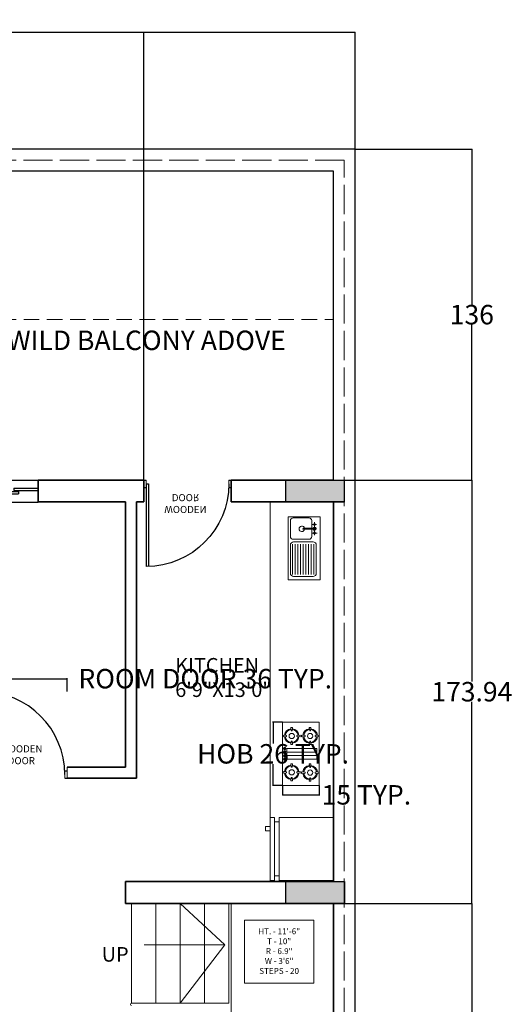
# Model space of a CAD drawing. Units: inches. Extents: x -48 to 50072, y 0 to 21068.
# Tile 56 of 75: x 415 to 618, y 819 to 1224. Entities that reach past the tile are written whole.
import ezdxf

# ---------------------------------------------------------------- set-up
doc = ezdxf.new("R2010")
doc.units = ezdxf.units.IN
doc.header["$MEASUREMENT"] = 0
doc.linetypes.add('ACAD_ISO02W100', pattern=[15, 12, -3])
doc.linetypes.add('HIDDEN', pattern=[9.525, 6.35, -3.175])
for name, color, linetype, lineweight in [('A-ANNO-DIMS', 2, 'Continuous', 18), ('A-ANNO-SYMB', 7, 'Continuous', 18), ('A-ANNO-TEXT', 7, 'Continuous', 18), ('A-AREA-IDEN', 7, 'Continuous', 18), ('A-COLS', 1, 'Continuous', 35), ('A-DOOR', 4, 'Continuous', 18), ('A-EQPM', 8, 'Continuous', 18), ('A-FLOR-CASE', 9, 'Continuous', 18), ('A-FLOR-FIXT', 4, 'Continuous', 18), ('A-FLOR-OVHD', 8, 'HIDDEN', 13), ('A-FLOR-STRS', 7, 'Continuous', 18), ('A-GLAZ', 4, 'Continuous', 18), ('A-WALL', 7, 'Continuous', 35), ('C-PROP', 7, 'Continuous', 25), ('C-PROP-REF', 32, 'ACAD_ISO02W100', 13)]:
    doc.layers.add(name, color=color, linetype=linetype, lineweight=lineweight)
doc.layers.add('Layer3', color=176, linetype='Continuous')
doc.styles.get("Standard").update_dxf_attribs({"font": 'arial.ttf'})
doc.dimstyles.get("Standard").update_dxf_attribs({"dimtxt": 8, "dimasz": 0.18, "dimexe": 0.18, "dimexo": 0.0625, "dimgap": 0.09, "dimtad": 0, "dimtih": 1, "dimtoh": 1, "dimdec": 1, "dimzin": 0, "dimdsep": 46, "dimlunit": 4, "dimtxsty": 'Standard', "dimblk": 'ARCHTICK', "dimcen": 0.09, "dimadec": 0, "dimazin": 0, "dimtfac": 1, "dimtdec": 1, "dimtofl": 0, "dimtmove": 0, "dimatfit": 3, "dimldrblk": 'ARCHTICK', "dimfxl": 1, "dimtolj": 1, "dimtzin": 0, "dimarcsym": 0})

# ---------------------------------------------------------------- blocks, each defined once
blk = doc.blocks.new('bnniku')
at = {"layer": 'Defpoints'}
h = blk.add_hatch(color=256, dxfattribs=at)
h.dxf.hatch_style = 1
h.paths.add_polyline_path([(767.55, 1114.04), (758.55, 1114.04), (758.55, 1090.04), (767.55, 1090.04)])
for p, q in [((758.55, 1114.04), (767.55, 1114.04)), ((758.55, 1090.04), (758.55, 1114.04)), ((767.55, 1114.04), (767.55, 1090.04)), ((767.55, 1090.04), (758.55, 1090.04))]:
    blk.add_line(p, q, dxfattribs=at)
blk = doc.blocks.new('jyugcli')
for p, q in [((342.02, 1025.77), (342.02, 1034.77)), ((360.02, 1025.77), (360.02, 1034.77))]:
    blk.add_line(p, q)
at = {"layer": 'Defpoints'}
for p, q in [((342.02, 1030.07), (352.02, 1030.07)), ((342.02, 1029.07), (352.02, 1029.07)), ((350.02, 1031.47), (360.02, 1031.47)), ((350.02, 1031.47), (350.02, 1030.47)), ((350.02, 1030.47), (360.02, 1030.47)), ((352.02, 1030.07), (352.02, 1029.07))]:
    blk.add_line(p, q, dxfattribs=at)
at = {"layer": 'Layer3'}
for p, q in [((342.02, 1034.77), (360.02, 1034.77)), ((342.02, 1025.77), (360.02, 1025.77))]:
    blk.add_line(p, q, dxfattribs=at)
blk = doc.blocks.new('BKUHJKKUG')
at = {"layer": 'Defpoints'}
for p, q in [((179.52, 862.77), (179.52, 896.77)), ((180.52, 862.77), (180.52, 896.76)), ((179.52, 862.77), (180.52, 862.77))]:
    blk.add_line(p, q, dxfattribs=at)
blk.add_arc((179.52, 862.77), 34, 0, 90, dxfattribs=at)
at = {"insert": (190.84, 874.8), "char_height": 2.9183, "attachment_point": 1}
blk.add_mtext_dynamic_manual_height_columns('\\pxqc;WOODEN ^JDOOR', width=9.6242, gutter_width=14.59, heights=[0], dxfattribs=at)
blk = doc.blocks.new('yfhjudru')
for p, q in [((399.02, 912.27), (399.02, 916.77)), ((400.02, 912.27), (400.02, 915.27)), ((434.02, 912.27), (434.02, 915.27)), ((435.02, 912.27), (435.02, 916.77))]:
    blk.add_line(p, q)
at = {"layer": 'Defpoints'}
for p, q in [((399.02, 915.27), (400.02, 915.27)), ((434.02, 915.27), (435.02, 915.27)), ((399.02, 912.27), (400.02, 912.27)), ((434.02, 912.27), (435.02, 912.27))]:
    blk.add_line(p, q, dxfattribs=at)
blk.add_blockref('BKUHJKKUG', (220.5, 51), dxfattribs=at)
blk = doc.blocks.new('A$C593E77E4')
for p, q in [((0, 0), (0, 0.911)), ((0, 0.911), (1.781, 0.911)), ((1.781, 0), (1.781, 0.911)), ((0.03, 0.593), (0.03, 0.141)), ((0.321, 0.668), (0.105, 0.668)), ((0.279, 0.745, -0.922), (0.15, 0.745, -0.922)), ((0.216, 0.808, -0.922), (0.216, 0.672, -0.922)), ((0.321, 0.784, -0.922), (0.321, 0.434, -0.922)), ((0.349, 0.784, -0.922), (0.321, 0.784, -0.922)), ((0.349, 0.434, -0.922), (0.349, 0.784, -0.922)), ((0.555, 0.668), (0.349, 0.668)), ((0.39, 0.745, -0.922), (0.519, 0.745, -0.922)), ((0.455, 0.826, -0.922), (0.455, 0.689, -0.922)), ((0.63, 0.141), (0.63, 0.593)), ((0.705, 0.706), (0.705, 0.158)), ((0.772, 0.729, 1.373), (1.625, 0.729, 1.373)), ((0.772, 0.654, 1.373), (1.625, 0.654, 1.373)), ((0.772, 0.579, 1.373), (1.625, 0.579, 1.373)), ((1.588, 0.797), (0.797, 0.797)), ((1.68, 0.158), (1.68, 0.706)), ((0.772, 0.504, 1.373), (1.625, 0.504, 1.373)), ((0.772, 0.429, 1.373), (1.625, 0.429, 1.373)), ((0.772, 0.354, 1.373), (1.625, 0.354, 1.373)), ((0.772, 0.279, 1.373), (1.625, 0.279, 1.373)), ((0.105, 0.066), (0.555, 0.066)), ((0.772, 0.204, 1.373), (1.625, 0.204, 1.373)), ((0.772, 0.129, 1.373), (1.625, 0.129, 1.373)), ((0.797, 0.066), (1.588, 0.066)), ((1.781, 0), (0, 0))]:
    blk.add_line(p, q)
for centre in [(0.216, 0.745, -0.922), (0.454, 0.745, -0.922)]:
    blk.add_circle(centre, 0.0299)
for centre, radius, start, end in [((0.105, 0.593), 0.075, 90, 180), ((0.333, 0.75, -0.922), 0.0447, 290.1713, 253.9866), ((0.555, 0.593), 0.075, 0, 90), ((0.797, 0.706), 0.0919, 90, 180), ((1.588, 0.706), 0.0919, 0, 90), ((0.336, 0.387, 0.688), 0.0774, 101.239, 83.3158), ((0.335, 0.435, -0.922), 0.0139, 185.1203, 354.8797), ((0.105, 0.141), 0.075, 180, 270), ((0.555, 0.141), 0.075, 270, 0), ((0.797, 0.158), 0.0919, 180, 270), ((1.588, 0.158), 0.0919, 270, 0)]:
    blk.add_arc(centre, radius, start, end)
blk = doc.blocks.new('A$C57CF26DA')
for p, q in [((0, 0), (0, 420)), ((720, 420), (0, 420)), ((167, 413), (147, 413)), ((147, 413), (152, 373)), ((152, 373), (162, 373)), ((162, 373), (167, 413)), ((300, 391), (300, 49)), ((300, 391), (420, 391)), ((340, 391), (340, 49)), ((380, 391), (380, 49)), ((420, 391), (420, 49)), ((584, 413), (564, 413)), ((564, 413), (569, 373)), ((569, 373), (579, 373)), ((579, 373), (584, 413)), ((720, 0), (720, 420)), ((99, 320), (59, 325)), ((59, 325), (59, 305)), ((59, 305), (99, 310)), ((99, 310), (99, 320)), ((152, 257), (147, 217)), ((162, 257), (152, 257)), ((167, 217), (162, 257)), ((255, 325), (215, 320)), ((215, 320), (215, 310)), ((215, 310), (255, 305)), ((255, 305), (255, 325)), ((516, 320), (476, 325)), ((476, 325), (476, 305)), ((476, 305), (516, 310)), ((516, 310), (516, 320)), ((569, 257), (564, 217)), ((579, 257), (569, 257)), ((584, 217), (579, 257)), ((672, 325), (632, 320)), ((632, 320), (632, 310)), ((632, 310), (672, 305)), ((672, 305), (672, 325)), ((99, 110), (59, 115)), ((59, 115), (59, 95)), ((147, 217), (167, 217)), ((167, 203), (147, 203)), ((147, 203), (152, 163)), ((152, 163), (162, 163)), ((162, 163), (167, 203)), ((255, 115), (215, 110)), ((255, 95), (255, 115)), ((513, 110), (473, 115)), ((473, 115), (473, 95)), ((581, 203), (561, 203)), ((561, 203), (566, 163)), ((564, 217), (584, 217)), ((566, 163), (576, 163)), ((576, 163), (581, 203)), ((669, 115), (629, 110)), ((669, 95), (669, 115)), ((59, 95), (99, 100)), ((99, 100), (99, 110)), ((152, 47), (147, 7)), ((147, 7), (167, 7)), ((162, 47), (152, 47)), ((167, 7), (162, 47)), ((215, 110), (215, 100)), ((215, 100), (255, 95)), ((302, 39), (295, 39)), ((295, 39), (295, 11)), ((295, 11), (302, 11)), ((420, 49), (300, 49)), ((302, 11), (302, 39)), ((341, 39), (334, 39)), ((334, 39), (334, 11)), ((334, 11), (341, 11)), ((341, 11), (341, 39)), ((380, 11), (380, 39)), ((380, 39), (386, 39)), ((386, 11), (380, 11)), ((386, 39), (386, 11)), ((419, 11), (419, 39)), ((419, 39), (426, 39)), ((426, 11), (419, 11)), ((426, 39), (426, 11)), ((473, 95), (513, 100)), ((513, 100), (513, 110)), ((566, 47), (561, 7)), ((561, 7), (581, 7)), ((576, 47), (566, 47)), ((581, 7), (576, 47)), ((629, 110), (629, 100)), ((629, 100), (669, 95)), ((720, 0), (0, 0))]:
    blk.add_line(p, q)
for centre in [(157, 315), (574, 315), (157, 105), (571, 105)]:
    blk.add_circle(centre, 30)
for centre, radius, start, end in [((157, 315), 83, 95.5849, 174.4151), ((157, 315), 73, 95.3738, 174.6262), ((157, 315), 73, 5.3738, 84.6262), ((157, 315), 83, 5.5849, 84.4151), ((574, 315), 83, 95.5849, 174.4151), ((574, 315), 73, 95.3738, 174.6262), ((574, 315), 73, 5.3738, 84.6262), ((574, 315), 83, 5.5849, 84.4151), ((157, 315), 83, 185.5849, 264.4151), ((157, 315), 73, 185.3738, 264.6262), ((157, 315), 73, 275.3738, 354.6262), ((157, 315), 83, 275.5849, 354.4151), ((574, 315), 83, 185.5849, 264.4151), ((574, 315), 73, 185.3738, 264.6262), ((574, 315), 73, 275.3738, 354.6262), ((574, 315), 83, 275.5849, 354.4151), ((157, 105), 83, 95.5849, 174.4151), ((157, 105), 73, 95.3738, 174.6262), ((157, 105), 73, 5.3738, 84.6262), ((157, 105), 83, 5.5849, 84.4151), ((571, 105), 83, 95.5849, 174.4151), ((571, 105), 73, 95.3738, 174.6262), ((571, 105), 73, 5.3738, 84.6262), ((571, 105), 83, 5.5849, 84.4151), ((157, 105), 83, 185.5849, 264.4151), ((157, 105), 73, 185.3738, 264.6262), ((157, 105), 73, 275.3738, 354.6262), ((157, 105), 83, 275.5849, 354.4151), ((298, 25), 13.7, 104.4775, 255.5225), ((298, 25), 13.7, 284.4775, 75.5225), ((337, 25), 13.7, 104.4775, 255.5225), ((337, 25), 13.7, 284.4775, 75.5225), ((383, 25), 13.7, 104.4775, 255.5225), ((383, 25), 13.7, 284.4775, 75.5225), ((422, 25), 13.7, 104.4775, 255.5225), ((422, 25), 13.7, 284.4775, 75.5225), ((571, 105), 83, 185.5849, 264.4151), ((571, 105), 73, 185.3738, 264.6262), ((571, 105), 73, 275.3738, 354.6262), ((571, 105), 83, 275.5849, 354.4151)]:
    blk.add_arc(centre, radius, start, end)
blk = doc.blocks.new('REFRI-00')
for points in [[(-0.35, 0.35), (-0.35, -0.25), (0.35, -0.25), (0.35, 0.35), (-0.35, 0.35)], [(-0.35, -0.3), (-0.35, -0.35), (0.35, -0.35), (0.35, -0.3), (-0.35, -0.3)], [(-0.3, -0.3), (-0.3, -0.25)], [(0.3, -0.3), (0.3, -0.25)], [(-0.25, -0.35), (-0.25, -0.4), (-0.2, -0.4), (-0.2, -0.35)]]:
    blk.add_lwpolyline(points)
blk = doc.blocks.new('_ArchTick')
at = {"color": 0, "linetype": 'ByBlock', "const_width": 0.15}
blk.add_lwpolyline([(-0.5, -0.5), (0.5, 0.5)], dxfattribs=at)
blk = doc.blocks.new('*D64')
at = {"layer": 'A-ANNO-DIMS', "color": 0, "lineweight": -2, "transparency": 16777216}
for p, q in [((399.02, 947.84), (399.02, 953.35)), ((399.02, 953.17), (435.02, 953.17)), ((435.02, 947.84), (435.02, 953.35)), ((435.02, 953.17), (435.2, 953.17))]:
    blk.add_line(p, q, dxfattribs=at)
at = {"layer": 'Defpoints', "color": 0, "transparency": 16777216}
for p in [(435.02, 953.17), (399.02, 947.77), (435.02, 947.77)]:
    blk.add_point(p, dxfattribs=at)
at = {"layer": 'A-ANNO-DIMS', "color": 0, "lineweight": -2, "transparency": 16777216, "xscale": 0.18, "yscale": 0.18, "zscale": 0.18, "rotation": 180}
blk.add_blockref('_ArchTick', (399.02, 953.17), dxfattribs=at)
at = {"layer": 'A-ANNO-DIMS', "color": 0, "lineweight": -2, "transparency": 16777216, "xscale": 0.18, "yscale": 0.18, "zscale": 0.18}
blk.add_blockref('_ArchTick', (435.02, 953.17), dxfattribs=at)
at = {"layer": 'A-ANNO-DIMS', "color": 0, "transparency": 16777216, "insert": (491.8, 953.17), "char_height": 8, "attachment_point": 5}
blk.add_mtext('\\A1;ROOM DOOR 36 TYP.', dxfattribs=at)
blk = doc.blocks.new('*D90')
at = {"layer": 'A-ANNO-DIMS', "color": 0, "lineweight": -2, "transparency": 16777216}
for p, q in [((523.53, 935.26), (519.52, 935.26)), ((519.7, 935.26), (519.7, 926.52)), ((519.7, 909.32), (519.7, 918.06)), ((523.53, 909.32), (519.52, 909.32))]:
    blk.add_line(p, q, dxfattribs=at)
at = {"layer": 'Defpoints', "color": 0, "transparency": 16777216}
for p in [(523.59, 935.26), (519.7, 909.32), (523.59, 909.32)]:
    blk.add_point(p, dxfattribs=at)
at = {"layer": 'A-ANNO-DIMS', "color": 0, "lineweight": -2, "transparency": 16777216, "xscale": 0.18, "yscale": 0.18, "zscale": 0.18}
for p, rotation in [((519.7, 935.26), 90), ((519.7, 909.32), 270)]:
    blk.add_blockref('_ArchTick', p, dxfattribs=dict(at, rotation=rotation))
at = {"layer": 'A-ANNO-DIMS', "color": 0, "transparency": 16777216, "insert": (519.7, 922.29), "char_height": 8, "attachment_point": 5}
blk.add_mtext('\\A1;HOB 26 TYP.', dxfattribs=at)
blk = doc.blocks.new('*D91')
at = {"layer": 'A-ANNO-DIMS', "color": 0, "lineweight": -2, "transparency": 16777216}
for p, q in [((523.59, 909.26), (523.59, 905.25)), ((538.73, 909.26), (538.73, 905.25)), ((523.59, 905.43), (538.73, 905.43)), ((538.73, 905.43), (538.91, 905.43))]:
    blk.add_line(p, q, dxfattribs=at)
at = {"layer": 'Defpoints', "color": 0, "transparency": 16777216}
for p in [(523.59, 909.32), (538.73, 909.32), (538.73, 905.43)]:
    blk.add_point(p, dxfattribs=at)
at = {"layer": 'A-ANNO-DIMS', "color": 0, "lineweight": -2, "transparency": 16777216, "xscale": 0.18, "yscale": 0.18, "zscale": 0.18, "rotation": 180}
blk.add_blockref('_ArchTick', (523.59, 905.43), dxfattribs=at)
at = {"layer": 'A-ANNO-DIMS', "color": 0, "lineweight": -2, "transparency": 16777216, "xscale": 0.18, "yscale": 0.18, "zscale": 0.18}
blk.add_blockref('_ArchTick', (538.73, 905.43), dxfattribs=at)
at = {"layer": 'A-ANNO-DIMS', "color": 0, "transparency": 16777216, "insert": (558.09, 905.43), "char_height": 8, "attachment_point": 5}
blk.add_mtext('\\A1;15 TYP.', dxfattribs=at)
blk = doc.blocks.new('*D112')
at = {"layer": 'A-ANNO-DIMS', "color": 0, "lineweight": -2, "transparency": 16777216}
for p, q in [((13.52, 1170.84), (13.52, 1218.9)), ((13.52, 1218.72), (274.6, 1218.72)), ((553.52, 1218.72), (292.43, 1218.72)), ((553.52, 1170.84), (553.52, 1218.9))]:
    blk.add_line(p, q, dxfattribs=at)
at = {"layer": 'Defpoints', "color": 0, "transparency": 16777216}
for p in [(553.52, 1218.72), (13.52, 1170.77), (553.52, 1170.77)]:
    blk.add_point(p, dxfattribs=at)
at = {"layer": 'A-ANNO-DIMS', "color": 0, "lineweight": -2, "transparency": 16777216, "xscale": 0.18, "yscale": 0.18, "zscale": 0.18, "rotation": 180}
blk.add_blockref('_ArchTick', (13.52, 1218.72), dxfattribs=at)
at = {"layer": 'A-ANNO-DIMS', "color": 0, "lineweight": -2, "transparency": 16777216, "xscale": 0.18, "yscale": 0.18, "zscale": 0.18}
blk.add_blockref('_ArchTick', (553.52, 1218.72), dxfattribs=at)
at = {"layer": 'A-ANNO-DIMS', "color": 0, "transparency": 16777216, "insert": (283.52, 1218.72), "char_height": 8, "attachment_point": 5}
blk.add_mtext('\\A1;540', dxfattribs=at)
blk = doc.blocks.new('*D114')
at = {"layer": 'A-ANNO-DIMS', "color": 0, "lineweight": -2, "transparency": 16777216}
for p, q in [((553.58, 1170.77), (601.65, 1170.77)), ((601.47, 1170.77), (601.47, 1106.95)), ((601.47, 1034.77), (601.47, 1098.6)), ((549.08, 1034.77), (601.65, 1034.77))]:
    blk.add_line(p, q, dxfattribs=at)
at = {"layer": 'Defpoints', "color": 0, "transparency": 16777216}
for p in [(553.52, 1170.77), (549.02, 1034.77), (601.47, 1034.77)]:
    blk.add_point(p, dxfattribs=at)
at = {"layer": 'A-ANNO-DIMS', "color": 0, "lineweight": -2, "transparency": 16777216, "xscale": 0.18, "yscale": 0.18, "zscale": 0.18}
for p, rotation in [((601.47, 1170.77), 90), ((601.47, 1034.77), 270)]:
    blk.add_blockref('_ArchTick', p, dxfattribs=dict(at, rotation=rotation))
at = {"layer": 'A-ANNO-DIMS', "color": 0, "transparency": 16777216, "insert": (601.47, 1102.77), "char_height": 8, "attachment_point": 5}
blk.add_mtext('\\A1;136', dxfattribs=at)
blk = doc.blocks.new('*D120')
at = {"layer": 'A-ANNO-DIMS', "color": 0, "lineweight": -2, "transparency": 16777216}
for p, q in [((549.08, 1034.77), (601.65, 1034.77)), ((601.47, 1034.77), (601.47, 951.98)), ((601.47, 860.84), (601.47, 943.63)), ((549.08, 860.84), (601.65, 860.84))]:
    blk.add_line(p, q, dxfattribs=at)
at = {"layer": 'Defpoints', "color": 0, "transparency": 16777216}
for p in [(549.02, 1034.77), (549.02, 860.84), (601.47, 860.84)]:
    blk.add_point(p, dxfattribs=at)
at = {"layer": 'A-ANNO-DIMS', "color": 0, "lineweight": -2, "transparency": 16777216, "xscale": 0.18, "yscale": 0.18, "zscale": 0.18}
for p, rotation in [((601.47, 1034.77), 90), ((601.47, 860.84), 270)]:
    blk.add_blockref('_ArchTick', p, dxfattribs=dict(at, rotation=rotation))
at = {"layer": 'A-ANNO-DIMS', "color": 0, "transparency": 16777216, "insert": (601.47, 947.81), "char_height": 8, "attachment_point": 5}
blk.add_mtext('\\A1;173.94', dxfattribs=at)
blk = doc.blocks.new('*D121')
at = {"layer": 'A-ANNO-DIMS', "color": 0, "lineweight": -2, "transparency": 16777216}
for p, q in [((549.08, 860.84), (601.65, 860.84)), ((601.47, 860.84), (601.47, 777.98)), ((601.47, 686.77), (601.47, 769.63)), ((549.08, 686.77), (601.65, 686.77))]:
    blk.add_line(p, q, dxfattribs=at)
at = {"layer": 'Defpoints', "color": 0, "transparency": 16777216}
for p in [(549.02, 860.84), (549.02, 686.77), (601.47, 686.77)]:
    blk.add_point(p, dxfattribs=at)
at = {"layer": 'A-ANNO-DIMS', "color": 0, "lineweight": -2, "transparency": 16777216, "xscale": 0.18, "yscale": 0.18, "zscale": 0.18}
for p, rotation in [((601.47, 860.84), 90), ((601.47, 686.77), 270)]:
    blk.add_blockref('_ArchTick', p, dxfattribs=dict(at, rotation=rotation))
at = {"layer": 'A-ANNO-DIMS', "color": 0, "transparency": 16777216, "insert": (601.47, 773.81), "char_height": 8, "attachment_point": 5}
blk.add_mtext('\\A1;174.06', dxfattribs=at)
blk = doc.blocks.new('*D124')
at = {"layer": 'A-ANNO-DIMS', "color": 0, "lineweight": -2, "transparency": 16777216}
for p, q in [((297.02, 1034.84), (297.02, 1218.9)), ((297.02, 1218.72), (368.53, 1218.72)), ((466.52, 1218.72), (395.01, 1218.72)), ((466.52, 1034.84), (466.52, 1218.9))]:
    blk.add_line(p, q, dxfattribs=at)
at = {"layer": 'Defpoints', "color": 0, "transparency": 16777216}
for p in [(466.52, 1218.72), (297.02, 1034.77), (466.52, 1034.77)]:
    blk.add_point(p, dxfattribs=at)
at = {"layer": 'A-ANNO-DIMS', "color": 0, "lineweight": -2, "transparency": 16777216, "xscale": 0.18, "yscale": 0.18, "zscale": 0.18, "rotation": 180}
blk.add_blockref('_ArchTick', (297.02, 1218.72), dxfattribs=at)
at = {"layer": 'A-ANNO-DIMS', "color": 0, "lineweight": -2, "transparency": 16777216, "xscale": 0.18, "yscale": 0.18, "zscale": 0.18}
blk.add_blockref('_ArchTick', (466.52, 1218.72), dxfattribs=at)
at = {"layer": 'A-ANNO-DIMS', "color": 0, "transparency": 16777216, "insert": (381.77, 1218.72), "char_height": 8, "attachment_point": 5}
blk.add_mtext('\\A1;169.5', dxfattribs=at)

msp = doc.modelspace()

# ---------------------------------------------------------------- linework, layer by layer
at = {"layer": 'A-ANNO-SYMB'}
for p, q in [((499.798, 843.778), (481.517, 860.838)), ((466.695, 843.778), (499.798, 843.778)), ((499.798, 843.778), (481.517, 819.838))]:
    msp.add_line(p, q, dxfattribs=at)
at = {"layer": 'A-ANNO-TEXT'}
msp.add_lwpolyline([(508.007, 853.988), (536.464, 853.988), (536.464, 828.07), (508.007, 828.07)], close=True, dxfattribs=at)
at = {"layer": 'A-FLOR-CASE'}
msp.add_line((518.517, 869.775), (518.517, 1025.775), dxfattribs=at)
at = {"layer": 'A-FLOR-OVHD'}
msp.add_line((360.017, 1100.775), (544.517, 1100.775), dxfattribs=at)
at = {"layer": 'A-FLOR-STRS'}
for p, q in [((461.517, 819.838), (461.517, 860.838)), ((471.517, 819.838), (471.517, 860.838)), ((481.517, 819.838), (481.517, 860.838)), ((491.517, 819.838), (491.517, 860.838)), ((501.517, 819.838), (501.517, 860.838)), ((502.517, 768.838), (502.517, 860.838)), ((501.517, 819.838), (461.517, 819.838))]:
    msp.add_line(p, q, dxfattribs=at)
msp.add_arc((461.517, 819.338), 0.5, 90, 270, dxfattribs=at)
at = {"layer": 'A-WALL'}
for p, q in [((423.017, 1025.775), (423.017, 1034.775)), ((466.517, 1034.775), (423.017, 1034.775)), ((466.517, 1025.775), (466.517, 1034.775)), ((544.517, 1034.775), (502.517, 1034.775)), ((502.517, 1025.775), (502.517, 1034.775)), ((459.017, 1025.775), (423.017, 1025.775)), ((459.017, 916.775), (459.017, 1025.775)), ((463.517, 912.275), (463.517, 1025.775)), ((466.517, 1025.775), (463.517, 1025.775)), ((549.017, 1025.775), (502.517, 1025.775)), ((544.517, 869.775), (544.517, 1025.775)), ((459.017, 916.775), (435.017, 916.775)), ((463.517, 912.275), (435.017, 912.275)), ((544.517, 869.775), (459.017, 869.775)), ((459.017, 860.775), (459.017, 869.775)), ((549.017, 860.838), (459.017, 860.838)), ((544.517, 686.775), (544.517, 860.838))]:
    msp.add_line(p, q, dxfattribs=at)
at = {"layer": 'C-PROP'}
for p, q in [((553.517, 1170.775), (13.517, 1170.775)), ((553.517, 214.075), (553.517, 1170.775)), ((544.517, 1161.775), (22.517, 1161.775)), ((544.517, 1034.775), (544.517, 1161.775))]:
    msp.add_line(p, q, dxfattribs=at)
at = {"layer": 'C-PROP-REF'}
for p, q in [((549.017, 1166.275), (18.017, 1166.275)), ((549.017, 214.075), (549.017, 1166.275))]:
    msp.add_line(p, q, dxfattribs=at)

# ---------------------------------------------------------------- block references
at = {"layer": 'A-COLS'}
for p, rotation in [((1639.054, 267.223), 90), ((-565.02, 1628.39), 270)]:
    msp.add_blockref('bnniku', p, dxfattribs=dict(at, rotation=rotation))
at = {"layer": 'A-DOOR', "xscale": -1, "rotation": 180}
msp.add_blockref('yfhjudru', (67.5, 1947.05), dxfattribs=at)
at = {"layer": 'A-DOOR'}
msp.add_blockref('yfhjudru', (0, 0), dxfattribs=at)
at = {"layer": 'A-EQPM', "rotation": 270}
for name, p, xscale, yscale, zscale in [('A$C57CF26DA', (523.594, 935.262), 0.0360302478784816, 0.0360302478784816, 0.0360302478784816), ('REFRI-00', (531.427, 883.202), 36.94664574988657, 36.94664574988657, 36.94664574988657)]:
    msp.add_blockref(name, p, dxfattribs=dict(at, xscale=xscale, yscale=yscale, zscale=zscale))
at = {"layer": 'A-FLOR-FIXT', "xscale": 14.56160544363934, "yscale": 14.56160544363934, "zscale": 14.56160544363934, "rotation": 270}
msp.add_blockref('A$C593E77E4', (525.87, 1019.656), dxfattribs=at)
at = {"layer": 'A-GLAZ'}
msp.add_blockref('jyugcli', (63, 0), dxfattribs=at)

# ---------------------------------------------------------------- texts
at = {"layer": 'A-ANNO-SYMB', "insert": (449.211, 842.888), "char_height": 6, "attachment_point": 1}
msp.add_mtext_dynamic_manual_height_columns('UP', width=19.39027, gutter_width=30, heights=[0], dxfattribs=at)
at = {"layer": 'A-ANNO-TEXT', "attachment_point": 1}
for s, width, gutter_width, insert, char_height in [('4\'- 6" WILD BALCONY ADOVE ', 220.65422, 40, (381.401, 1096.216), 8), ('\\pxqc;HT. - 11\'-6"^JT - 10"^JR - 6.9"^JW - 3\'6"^JSTEPS - 20', 39.17224, 12.199, (502.616, 850.564), 2.4397)]:
    msp.add_mtext_dynamic_manual_height_columns(s, width=width, gutter_width=gutter_width, heights=[0], dxfattribs=dict(at, insert=insert, char_height=char_height))
at = {"layer": 'A-AREA-IDEN', "insert": (479.452, 961.657), "char_height": 6, "attachment_point": 1}
msp.add_mtext_dynamic_manual_height_columns('KITCHEN^J6\'9"X13\'0"', width=151.64395, gutter_width=30, heights=[0], dxfattribs=at)

# ---------------------------------------------------------------- dimensions: what is measured, and where the dimension line sits
at = {"layer": 'A-ANNO-DIMS'}
for base, p1, p2, override, picture, middle in [((553.517, 1218.725), (13.517, 1170.775), (553.517, 1170.775), {"dimdec": 0, "dimlfac": 1, "dimrnd": 0, "dimzin": 0, "dimdsep": 46, "dimlunit": 2}, '*D112', (283.517, 1218.725)), ((466.517, 1218.725), (297.017, 1034.775), (466.517, 1034.775), {"dimdec": 1, "dimlfac": 1, "dimrnd": 0, "dimzin": 0, "dimdsep": 46, "dimlunit": 2}, '*D124', (381.767, 1218.725))]:
    dim = msp.add_linear_dim(base=base, p1=p1, p2=p2, dimstyle='Standard', override=override, dxfattribs=at)
    dim.commit()
    dim.dimension.update_dxf_attribs({"geometry": picture, "text_midpoint": middle})
for base, p1, p2, override, picture, middle in [((601.467, 1034.775), (553.517, 1170.775), (549.017, 1034.775), {"dimdec": 0, "dimlfac": 1, "dimrnd": 0, "dimzin": 0, "dimdsep": 46, "dimlunit": 2}, '*D114', (601.467, 1102.775)), ((601.467, 860.838), (549.017, 1034.775), (549.017, 860.838), {"dimdec": 2, "dimlfac": 1, "dimrnd": 0, "dimzin": 0, "dimdsep": 46, "dimlunit": 2}, '*D120', (601.467, 947.806)), ((601.467, 686.775), (549.017, 860.838), (549.017, 686.775), {"dimdec": 2, "dimlfac": 1, "dimrnd": 0, "dimzin": 0, "dimdsep": 46, "dimlunit": 2}, '*D121', (601.467, 773.806))]:
    dim = msp.add_linear_dim(base=base, p1=p1, p2=p2, angle=90, dimstyle='Standard', override=override, dxfattribs=at)
    dim.commit()
    dim.dimension.update_dxf_attribs({"geometry": picture, "text_midpoint": middle})
for base, p1, p2, text, picture, middle in [((435.017, 953.175), (399.017, 947.775), (435.017, 947.775), 'ROOM DOOR <> TYP.', '*D64', (491.803, 953.175)), ((538.727, 905.429), (523.594, 909.32), (538.727, 909.32), '<> TYP.', '*D91', (558.091, 905.429))]:
    dim = msp.add_linear_dim(base=base, p1=p1, p2=p2, text=text, dimstyle='Standard', override={"dimdec": 0, "dimlfac": 1, "dimrnd": 0, "dimzin": 0, "dimdsep": 46, "dimlunit": 2}, dxfattribs=at)
    dim.commit()
    dim.dimension.update_dxf_attribs({"geometry": picture, "text_midpoint": middle})
dim = msp.add_linear_dim(base=(519.703, 909.32), p1=(523.594, 935.262), p2=(523.594, 909.32), angle=270, text='HOB <> TYP.', dimstyle='Standard', override={"dimdec": 0, "dimlfac": 1, "dimrnd": 0, "dimzin": 0, "dimdsep": 46, "dimlunit": 2}, dxfattribs=at)
dim.commit()
dim.dimension.update_dxf_attribs({"geometry": '*D90', "text_midpoint": (519.703, 922.291)})

doc.saveas('drawing.dxf')
